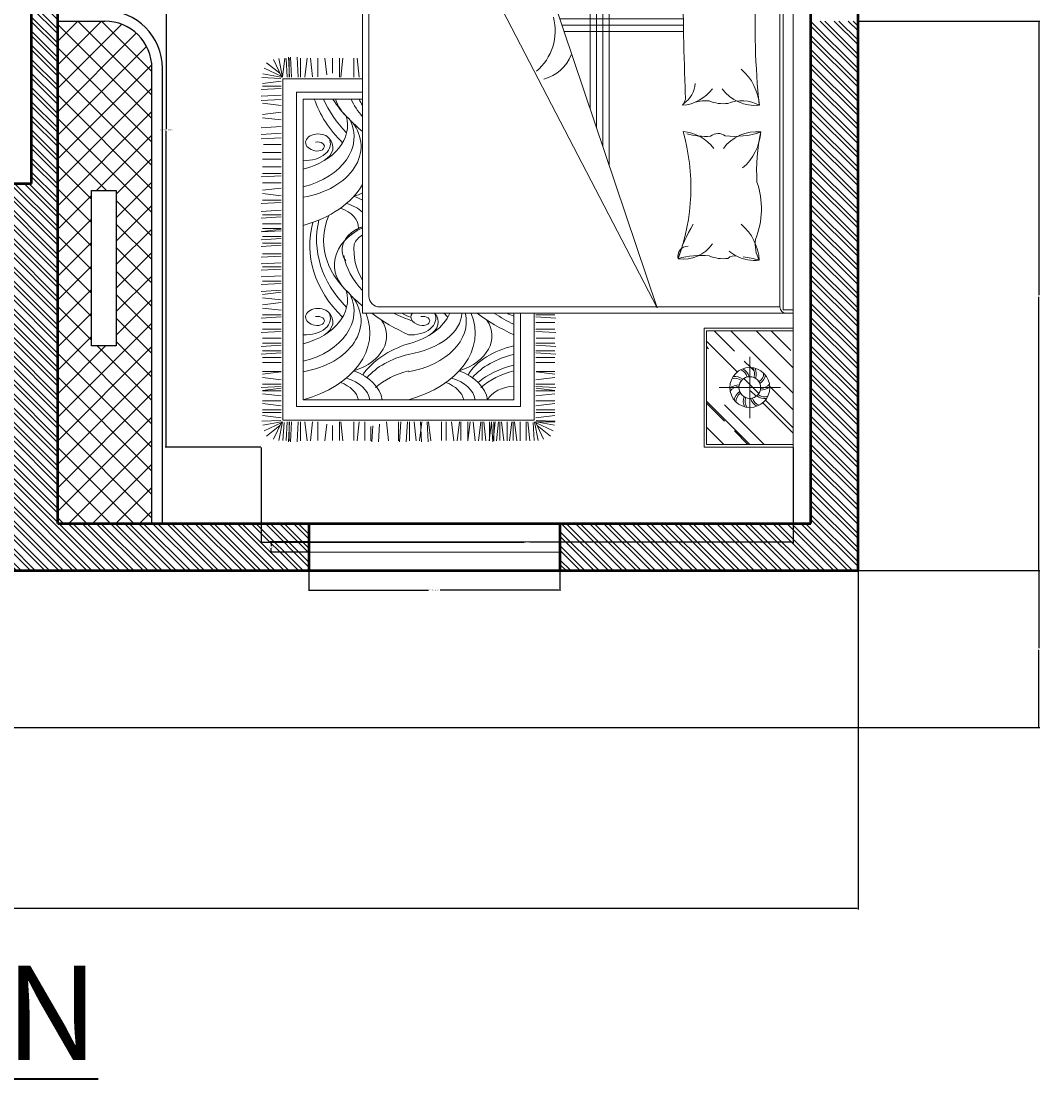
# Model space of a CAD drawing. Units: inches. Extents: x 10696 to 11614, y 5787 to 6498.
# Tile 2 of 9: x 10898 to 11093, y 5790 to 5992. Entities that reach past the tile are written whole.
import ezdxf

# ---------------------------------------------------------------- set-up
doc = ezdxf.new("R2010")
doc.units = ezdxf.units.IN
for name, color, linetype, lineweight in [('A-ANNO-DIMS', 2, 'Continuous', 18), ('A-ANNO-TITL', 7, 'Continuous', 35), ('A-FLOR-CASE', 32, 'Continuous', 25), ('A-FLOR-CASE-PATT', 252, 'Continuous', 13), ('A-FURN', 8, 'Continuous', 18), ('A-GLAZ', 4, 'Continuous', 20), ('A-WALL', 7, 'Continuous', 50), ('A-WALL-PATT', 252, 'Continuous', 13)]:
    doc.layers.add(name, color=color, linetype=linetype, lineweight=lineweight)
doc.styles.get("Standard").update_dxf_attribs({"font": 'arial.ttf'})
doc.dimstyles.get("Standard").update_dxf_attribs({"dimtxt": 0.18, "dimasz": 0.18, "dimexe": 0.18, "dimexo": 0.0625, "dimgap": 0.09, "dimtad": 0, "dimtih": 1, "dimtoh": 1, "dimdec": 4, "dimzin": 0, "dimdsep": 46, "dimtxsty": 'Standard', "dimcen": 0.09, "dimadec": 0, "dimazin": 0, "dimtfac": 1, "dimtdec": 4, "dimtofl": 0, "dimtmove": 0, "dimatfit": 3, "dimfxl": 1, "dimtolj": 1, "dimtzin": 0, "dimarcsym": 0})

# ---------------------------------------------------------------- blocks, each defined once
blk = doc.blocks.new('A$C64B41DC1')
for p, q in [((0, 2.5079), (2.9903, 2.5079)), ((0, 2.0879), (0, 2.5079)), ((0.012, 2.4618), (0.0581, 2.5079)), ((0.012, 2.3515), (0.1684, 2.5079)), ((0.012, 2.0999), (0.012, 2.5079)), ((0.0543, 2.2213), (0.3409, 2.5079)), ((0.1689, 2.4179), (0.2589, 2.5079)), ((0.3265, 2.386), (0.4484, 2.5079)), ((0.3699, 2.3332), (0.5445, 2.5079)), ((0.548, 2.5079), (0.548, 2.0999)), ((0.56, 2.5079), (0.56, 2.0879)), ((0.6301, 2.5079), (0.6301, 0.4779)), ((0.6401, 2.461), (0.6401, 2.5079)), ((0.6401, 2.5079), (2.344, 2.5079)), ((2.344, 2.5079), (2.3601, 2.5079)), ((2.344, 2.5079), (2.344, 2.461)), ((2.3601, 2.5079), (2.3601, 2.4761)), ((2.3601, 0.4779), (2.3601, 2.5079)), ((2.4303, 2.5079), (2.4303, 2.0879)), ((2.4423, 2.5079), (2.4423, 2.0999)), ((2.4423, 2.3333), (2.6169, 2.5079)), ((2.4423, 2.2145), (2.7357, 2.5079)), ((2.4423, 2.404), (2.5354, 2.4971)), ((2.705, 2.398), (2.8149, 2.5079)), ((2.7691, 2.3772), (2.8998, 2.5079)), ((2.7819, 2.3646), (2.9252, 2.5079)), ((2.9783, 2.0999), (2.9783, 2.5079)), ((2.9903, 2.0879), (2.9903, 2.5079)), ((0.2804, 2.1597), (0.2804, 2.4481)), ((2.344, 2.461), (0.6401, 2.461)), ((0.6601, 2.4461), (1.4951, 2.4461)), ((0.6601, 2.4461), (0.6601, 0.5579)), ((1.4951, 2.4461), (0.6697, 2.4461)), ((2.3301, 2.4461), (1.4951, 2.4461)), ((2.3301, 0.5579), (2.3301, 2.4461)), ((2.7099, 2.1597), (2.7099, 2.4481)), ((0.2157, 2.0999), (0.548, 2.4322)), ((0.2299, 2.0999), (0.548, 2.418)), ((0.2311, 2.2906), (0.2937, 2.3532)), ((2.6674, 2.2756), (2.7382, 2.3464)), ((2.7914, 2.1846), (2.9783, 2.3715)), ((0.1362, 2.3039), (0.4246, 2.3039)), ((0.2905, 2.2539), (0.3304, 2.2938)), ((0.3405, 2.3039), (0.3605, 2.3238)), ((2.8541, 2.3039), (2.5657, 2.3039)), ((2.5849, 2.2779), (2.6158, 2.3088)), ((2.6158, 2.3088), (2.6313, 2.3243)), ((2.7249, 2.3076), (2.7512, 2.3339)), ((2.7746, 2.0999), (2.9783, 2.3036)), ((2.9144, 2.2312), (2.9783, 2.2951)), ((0.012, 2.261), (0.0275, 2.2765)), ((0.0404, 2.0999), (0.1982, 2.2578)), ((2.4918, 2.0999), (2.6366, 2.2447)), ((0.1365, 2.0999), (0.251, 2.2144)), ((0.4194, 2.0999), (0.548, 2.2285)), ((2.4423, 2.1353), (2.5382, 2.2312)), ((0.4986, 2.0999), (0.548, 2.1493)), ((2.7831, 2.0999), (2.8678, 2.1846)), ((2.8962, 2.0999), (2.9783, 2.182)), ((0.548, 2.0999), (0.012, 2.0999)), ((0.5127, 2.0999), (0.548, 2.1352)), ((2.4423, 2.0999), (2.9783, 2.0999)), ((2.5172, 2.0999), (2.5269, 2.1096)), ((0.56, 2.0879), (0, 2.0879)), ((2.4303, 2.0879), (2.9903, 2.0879)), ((0.9415, 1.9902), (0.9415, 1.3975)), ((0.9715, 1.9906), (0.9715, 1.4076)), ((1.0015, 1.991), (1.0015, 1.4177)), ((1.0315, 1.9916), (1.0315, 1.4279)), ((2.3349, 1.8678), (0.6613, 1.3029)), ((0.8956, 1.1191), (2.3349, 1.8678)), ((1.6636, 1.6412), (0.6601, 1.6412)), ((1.5748, 1.6112), (0.6601, 1.6112)), ((2.3665, 1.295), (2.3665, 1.3839)), ((2.377, 1.295), (2.3822, 1.3891)), ((2.4032, 1.295), (2.4032, 1.3839)), ((2.4346, 1.295), (2.4346, 1.3839)), ((2.4451, 1.295), (2.4503, 1.3891)), ((2.4774, 1.2957), (2.4774, 1.3837)), ((2.5, 1.295), (2.5, 1.3839)), ((2.5105, 1.295), (2.5157, 1.3891)), ((2.5367, 1.295), (2.5367, 1.3839)), ((2.5471, 1.295), (2.5524, 1.3891)), ((2.5681, 1.295), (2.5681, 1.3839)), ((2.5918, 1.295), (2.5918, 1.3839)), ((2.6346, 1.2957), (2.6346, 1.3837)), ((2.6362, 1.2957), (2.6467, 1.3839)), ((2.6729, 1.295), (2.6624, 1.3839)), ((2.6938, 1.295), (2.6938, 1.3839)), ((2.7043, 1.295), (2.7095, 1.3891)), ((2.7127, 1.2957), (2.7232, 1.3839)), ((2.7253, 1.295), (2.7253, 1.3839)), ((2.7494, 1.295), (2.7389, 1.3839)), ((2.7718, 1.295), (2.7718, 1.3839)), ((2.7959, 1.295), (2.7854, 1.3839)), ((2.8146, 1.2957), (2.8146, 1.3837)), ((2.8146, 1.2957), (2.8146, 1.3837)), ((2.8282, 1.295), (2.8282, 1.3839)), ((2.8282, 1.295), (2.8282, 1.3839)), ((2.8523, 1.295), (2.8418, 1.3839)), ((2.8523, 1.295), (2.8418, 1.3839)), ((2.8653, 1.2966), (2.8688, 1.3861)), ((2.8711, 1.2957), (2.8711, 1.3837)), ((2.8711, 1.2957), (2.8875, 1.3822)), ((2.8765, 1.2958), (2.9132, 1.3758)), ((2.8893, 1.3011), (2.9394, 1.3636)), ((2.8713, 1.2927), (2.954, 1.3315)), ((2.8717, 1.2884), (2.9588, 1.3058)), ((2.3601, 1.2873), (2.8639, 1.2873)), ((2.8639, 1.2873), (2.8639, 0.1018)), ((2.8716, 1.2565), (2.9605, 1.2669)), ((2.8723, 1.2489), (2.9603, 1.2489)), ((2.8744, 1.2817), (2.9603, 1.2869)), ((2.3601, 1.2233), (2.7999, 1.2233)), ((2.7999, 1.2233), (2.7999, 0.1658)), ((2.8716, 1.2212), (2.9605, 1.2212)), ((2.8716, 1.1947), (2.9605, 1.2052)), ((2.3601, 1.1913), (2.7679, 1.1912)), ((2.7679, 1.1912), (2.7679, 0.1978)), ((2.8716, 1.181), (2.9605, 1.1705)), ((2.8716, 1.1595), (2.9605, 1.1595)), ((2.8723, 1.1872), (2.9603, 1.1872)), ((2.8716, 1.133), (2.9605, 1.1435)), ((2.8716, 1.1193), (2.9605, 1.1088)), ((2.8716, 1.1035), (2.9605, 1.093)), ((2.8723, 1.1255), (2.9603, 1.1255)), ((2.8716, 1.0965), (2.9605, 1.0965)), ((2.8716, 1.086), (2.9657, 1.0913)), ((2.8716, 1.0756), (2.9605, 1.0756)), ((2.8716, 1.0491), (2.9605, 1.0596)), ((2.8723, 1.0858), (2.9605, 1.0753)), ((2.8716, 1.0354), (2.9605, 1.0249)), ((2.8723, 1.0416), (2.9603, 1.0416)), ((2.8723, 0.9987), (2.9605, 1.0092)), ((2.8723, 0.985), (2.9605, 0.9745)), ((2.8723, 0.9735), (2.9603, 0.9735)), ((2.8716, 0.9346), (2.9605, 0.9241)), ((2.8723, 0.9408), (2.9603, 0.9408)), ((2.8723, 0.8979), (2.9605, 0.9084)), ((2.8723, 0.8726), (2.9603, 0.8726)), ((2.8723, 0.8505), (2.9603, 0.8505)), ((2.8716, 0.7885), (2.9605, 0.799)), ((2.8716, 0.7818), (2.9657, 0.787)), ((2.8716, 0.7503), (2.9657, 0.7556)), ((2.8723, 0.7571), (2.9605, 0.7466)), ((2.8716, 0.7204), (2.9605, 0.7309)), ((2.8716, 0.6995), (2.9605, 0.6995)), ((2.8716, 0.689), (2.9657, 0.6838)), ((2.8716, 0.6576), (2.9657, 0.6523)), ((2.8716, 0.6471), (2.9605, 0.6471)), ((2.8716, 0.5903), (2.9605, 0.6007)), ((2.882, 0.5582), (2.9657, 0.5536)), ((0.7101, 0.5079), (2.2801, 0.5079)), ((2.8909, 0.5263), (2.9657, 0.5222)), ((2.8928, 0.5169), (2.9605, 0.5169)), ((0.6301, 0.4779), (2.3601, 0.4779)), ((1.2465, 0.4625), (1.1576, 0.452)), ((1.2542, 0.1018), (1.2542, 0.4779)), ((1.3182, 0.1658), (1.3182, 0.4779)), ((1.3502, 0.1978), (1.3502, 0.4779)), ((2.8716, 0.4877), (2.9603, 0.4877)), ((2.8716, 0.4625), (2.9605, 0.452)), ((1.2465, 0.4365), (1.1577, 0.4365)), ((2.8716, 0.4365), (2.9603, 0.4365)), ((1.2465, 0.3746), (1.1576, 0.3851)), ((1.2465, 0.3684), (1.1577, 0.3684)), ((2.8716, 0.3746), (2.9605, 0.3851)), ((2.8716, 0.3684), (2.9603, 0.3684)), ((1.2355, 0.3092), (1.1576, 0.3)), ((1.2285, 0.3357), (1.1577, 0.3357)), ((2.8826, 0.3092), (2.9605, 0.3)), ((2.8896, 0.3357), (2.9603, 0.3357)), ((1.2457, 0.2676), (1.1577, 0.2676)), ((2.8723, 0.2676), (2.9603, 0.2676)), ((1.2457, 0.2423), (1.1576, 0.2319)), ((1.2465, 0.2057), (1.1576, 0.2161)), ((2.8716, 0.2057), (2.9605, 0.2161)), ((2.8723, 0.2423), (2.9605, 0.2319)), ((1.2465, 0.1742), (1.1524, 0.169)), ((1.2465, 0.1847), (1.1576, 0.1847)), ((2.7999, 0.1658), (1.3182, 0.1658)), ((2.7679, 0.1978), (1.3502, 0.1978)), ((2.8716, 0.1847), (2.9605, 0.1847)), ((2.8716, 0.1742), (2.9657, 0.169)), ((1.2465, 0.1428), (1.1524, 0.1376)), ((1.2465, 0.1334), (1.1524, 0.1281)), ((1.2465, 0.1323), (1.1576, 0.1323)), ((1.2465, 0.1323), (1.1576, 0.1323)), ((1.2465, 0.1), (1.1576, 0.1105)), ((1.2465, 0.1229), (1.1588, 0.1168)), ((1.2464, 0.1007), (1.1592, 0.0833)), ((2.8639, 0.1018), (1.2542, 0.1018)), ((2.8716, 0.1428), (2.9657, 0.1376)), ((2.8716, 0.1334), (2.9657, 0.1281)), ((2.8716, 0.1323), (2.9605, 0.1323)), ((2.8716, 0.1229), (2.9593, 0.1168)), ((2.8717, 0.1007), (2.9588, 0.0833)), ((2.8744, 0.1074), (2.9603, 0.1022)), ((1.2468, 0.0964), (1.1641, 0.0576)), ((1.2288, 0.088), (1.1787, 0.0255)), ((1.2415, 0.0933), (1.2049, 0.0133)), ((1.247, 0.0934), (1.2306, 0.0069)), ((1.2527, 0.0925), (1.2493, 0.003)), ((1.2658, 0.0941), (1.2762, 0.0052)), ((1.2899, 0.0941), (1.2899, 0.0052)), ((1.2999, 0.0941), (1.3051, 0)), ((1.3313, 0.0941), (1.3365, 0)), ((1.3523, 0.0941), (1.3575, 0)), ((1.3804, 0.0941), (1.3699, 0.0052)), ((1.4119, 0.0934), (1.4223, 0.0052)), ((1.4485, 0.0941), (1.438, 0.0052)), ((1.48, 0.0941), (1.4852, 0)), ((1.5114, 0.0941), (1.5166, 0)), ((1.5323, 0.0941), (1.5376, 0)), ((1.5638, 0.0941), (1.5638, 0.0105)), ((1.6021, 0.0941), (1.6021, 0.0052)), ((1.6336, 0.0941), (1.6336, 0.0052)), ((1.6702, 0.0941), (1.6702, 0.0052)), ((1.7017, 0.0941), (1.7017, 0.0052)), ((1.7122, 0.0941), (1.7174, 0)), ((1.7445, 0.0934), (1.7445, 0.0054)), ((1.7698, 0.0934), (1.7803, 0.0052)), ((1.8065, 0.0941), (1.796, 0.0052)), ((1.8274, 0.0941), (1.8274, 0.0052)), ((1.8379, 0.0941), (1.8431, 0)), ((1.8746, 0.0941), (1.8798, 0)), ((1.8955, 0.0941), (1.8955, 0.0052)), ((1.906, 0.0941), (1.9113, 0)), ((1.9384, 0.0934), (1.9384, 0.0054)), ((1.9609, 0.0941), (1.9609, 0.0052)), ((1.9636, 0.0934), (1.9741, 0.0052)), ((1.9714, 0.0941), (1.9766, 0)), ((1.9976, 0.0941), (1.9976, 0.0052)), ((2.0081, 0.0941), (2.0133, 0)), ((2.029, 0.0941), (2.029, 0.0052)), ((2.0395, 0.0941), (2.0447, 0)), ((2.0797, 0.0941), (2.0797, 0.0052)), ((2.0902, 0.0941), (2.0954, 0)), ((2.1216, 0.0941), (2.1269, 0)), ((2.1412, 0.0941), (2.1412, 0.0052)), ((2.1517, 0.0941), (2.1569, 0)), ((2.1831, 0.0941), (2.1884, 0)), ((2.2093, 0.0941), (2.2093, 0.0052)), ((2.2198, 0.0941), (2.225, 0)), ((2.2512, 0.0941), (2.2565, 0)), ((2.2603, 0.0934), (2.2707, 0.0052)), ((2.2969, 0.0941), (2.2864, 0.0052)), ((2.3089, 0.0934), (2.3193, 0.0052)), ((2.3455, 0.0941), (2.3351, 0.0052)), ((2.3665, 0.0941), (2.3665, 0.0052)), ((2.377, 0.0941), (2.3822, 0)), ((2.4032, 0.0941), (2.4032, 0.0052)), ((2.4346, 0.0941), (2.4346, 0.0052)), ((2.4451, 0.0941), (2.4503, 0)), ((2.4774, 0.0934), (2.4774, 0.0054)), ((2.5, 0.0941), (2.5, 0.0052)), ((2.5105, 0.0941), (2.5157, 0)), ((2.5367, 0.0941), (2.5367, 0.0052)), ((2.5471, 0.0941), (2.5524, 0)), ((2.5681, 0.0941), (2.5681, 0.0052)), ((2.5918, 0.0941), (2.5918, 0.0052)), ((2.6346, 0.0934), (2.6346, 0.0054)), ((2.6362, 0.0934), (2.6467, 0.0052)), ((2.6729, 0.0941), (2.6624, 0.0052)), ((2.6938, 0.0941), (2.6938, 0.0052)), ((2.7043, 0.0941), (2.7095, 0)), ((2.7127, 0.0934), (2.7232, 0.0052)), ((2.7253, 0.0941), (2.7253, 0.0052)), ((2.7494, 0.0941), (2.7389, 0.0052)), ((2.7718, 0.0941), (2.7718, 0.0052)), ((2.7959, 0.0941), (2.7854, 0.0052)), ((2.8146, 0.0934), (2.8146, 0.0054)), ((2.8282, 0.0941), (2.8282, 0.0052)), ((2.8523, 0.0941), (2.8418, 0.0052)), ((2.8653, 0.0925), (2.8688, 0.003)), ((2.8711, 0.0934), (2.8875, 0.0069)), ((2.8713, 0.0964), (2.954, 0.0576)), ((2.8765, 0.0933), (2.9132, 0.0133)), ((2.8893, 0.088), (2.9394, 0.0255))]:
    blk.add_line(p, q)
at = {"ltscale": 10}
for p, q in [((1.4859, 1.5812), (0.6601, 1.5812)), ((1.397, 1.5512), (0.6601, 1.5512))]:
    blk.add_line(p, q, dxfattribs=at)
for centre, radius in [((0.2804, 2.3039), 0.0942), ((2.7099, 2.3039), 0.0942), ((0.2804, 2.3039), 0.051), ((2.7099, 2.3039), 0.051)]:
    blk.add_circle(centre, radius)
for centre, radius, start, end in [((0.6601, 2.4761), 0.03, 180, 270), ((2.3301, 2.4761), 0.03, 270, 0), ((0.3286, 2.3561), 0.0605, 136.17, 182.4897), ((0.3231, 2.3585), 0.0462, 124.3002, 184.538), ((2.6672, 2.3585), 0.0462, 355.462, 55.6998), ((2.6617, 2.3561), 0.0605, 357.5103, 43.83), ((0.2417, 2.3614), 0.0462, 196.3002, 256.538), ((0.2887, 2.3745), 0.0605, 172.17, 218.4897), ((0.2828, 2.3731), 0.0462, 160.3002, 220.538), ((0.3501, 2.3178), 0.0605, 100.17, 146.4897), ((0.347, 2.323), 0.0462, 88.3002, 148.538), ((1.0526, 2.3302), 0.3085, 175.3048, 198.6942), ((-0.8702, 2.0941), 1.6364, 4.8098, 9.1892), ((0.8579, 2.6278), 0.2948, 247.5179, 264.267), ((0.728, 2.111), 0.245, 40.4189, 85.9871), ((1.0164, 5.7096), 3.3803, 266.8134, 276.1602), ((1.3963, 2.1044), 0.245, 94.0129, 139.5811), ((1.1858, 2.3288), 0.1943, 306.5711, 5.89), ((1.5348, 2.2652), 0.1767, 151.7736, 201.6983), ((1.6986, 2.3355), 0.1943, 174.11, 233.4289), ((1.1481, 2.2311), 0.3783, 353.4947, 19.1867), ((1.6871, 3.192), 0.8561, 257.7438, 273.6284), ((1.4882, 2.111), 0.245, 40.4189, 85.9871), ((1.8674, 1.9709), 0.3878, 68.2026, 108.9817), ((2.1269, 2.1044), 0.245, 94.0129, 139.5811), ((2.0342, 2.4856), 0.1563, 261.5958, 298.9092), ((1.9165, 2.3288), 0.1943, 333.7371, 5.89), ((2.6058, 2.2028), 0.517, 163.6046, 172.3273), ((2.6433, 2.323), 0.0462, 31.462, 91.6998), ((2.6402, 2.3178), 0.0605, 33.5103, 79.83), ((2.7075, 2.3731), 0.0462, 319.462, 19.6998), ((2.7016, 2.3745), 0.0605, 321.5103, 7.83), ((2.7486, 2.3614), 0.0462, 283.462, 343.6998), ((0.2457, 2.3659), 0.0605, 208.17, 254.4897), ((0.3449, 2.2742), 0.0605, 64.17, 110.4897), ((0.3455, 2.2802), 0.0462, 52.3002, 112.538), ((0.3151, 2.2419), 0.0605, 28.17, 74.4897), ((2.6448, 2.2802), 0.0462, 67.462, 127.6998), ((2.6454, 2.2742), 0.0605, 69.5103, 115.83), ((2.6752, 2.2419), 0.0605, 105.5103, 151.83), ((2.7446, 2.3659), 0.0605, 285.5103, 331.83), ((0.2153, 2.3276), 0.0462, 232.3002, 292.538), ((0.2158, 2.3336), 0.0605, 244.17, 290.4897), ((0.2138, 2.2848), 0.0462, 268.3002, 328.538), ((0.2107, 2.29), 0.0605, 280.17, 326.4897), ((0.2377, 2.2493), 0.0462, 304.3002, 4.538), ((0.2322, 2.2517), 0.0605, 316.17, 2.4897), ((0.2779, 2.2347), 0.0462, 340.3002, 40.538), ((0.272, 2.2333), 0.0605, 352.17, 38.4897), ((0.3191, 2.2464), 0.0462, 16.3002, 76.538), ((2.6712, 2.2464), 0.0462, 103.462, 163.6998), ((2.7182, 2.2333), 0.0605, 141.5103, 187.83), ((2.7123, 2.2347), 0.0462, 139.462, 199.6998), ((2.7581, 2.2517), 0.0605, 177.5103, 223.83), ((2.7526, 2.2493), 0.0462, 175.462, 235.6998), ((2.7796, 2.29), 0.0605, 213.5103, 259.83), ((2.7765, 2.2848), 0.0462, 211.462, 271.6998), ((2.7744, 2.3336), 0.0605, 249.5103, 295.83), ((2.775, 2.3276), 0.0462, 247.462, 307.6998), ((0.7274, 2.2013), 0.0446, 314.4736, 42.1713), ((-1.6008, 2.277), 2.3618, 357.3905, 358.8876), ((1.204, 2.1778), 0.1681, 337.017, 7.5368), ((1.9165, 2.3288), 0.1943, 320.9404, 333.7371), ((2.1347, 2.2313), 0.0459, 165.3506, 223.2684), ((1.9346, 2.1778), 0.1681, 337.017, 7.5368), ((0.2688, 2.0945), 0.4956, 344.0243, 8.7071), ((1.5671, 2.1546), 0.0547, 142.0833, 220.902), ((0.9385, 1.978), 0.1943, 126.5711, 185.89), ((1.1858, 1.9714), 0.1943, 4.3181, 53.4289), ((1.5415, 2.0969), 0.1834, 175.2233, 196.23), ((1.7059, 1.9714), 0.204, 127.1197, 175.09), ((1.1965, 2.0983), 0.3299, 343.7954, 3.5554), ((1.9394, 1.991), 0.1651, 351.2621, 55.7572), ((2.4617, 2.0719), 0.3745, 173.8296, 196.4356), ((1.2687, 1.9248), 0.1223, 33.628, 86.4744), ((0.7246, 18.8439), 16.8552, 270.17399, 272.05214), ((1.3401, 1.9404), 0.0603, 49.0991, 101.3702), ((1.7676, 1.0629), 0.9631, 69.6507, 105.9631), ((2.2748, 2.5795), 0.6373, 238.3499, 254.3137), ((2.0911, 2.0123), 0.0478, 179.7727, 283.8018), ((0.7417, 2.0149), 0.057, 273.4709, 328.5412), ((0.728, 2.2025), 0.245, 274.0129, 278.3417), ((1.0747, 1.2871), 0.1871, 14.1863, 69.1212), ((1.0274, 1.1334), 0.2527, 40.629, 104.3712), ((0.7347, 1.1553), 0.1649, 347.3109, 116.4454), ((0.7101, 0.5579), 0.05, 180, 270), ((2.2801, 0.5579), 0.05, 270, 0)]:
    blk.add_arc(centre, radius, start, end)
for centre, major_axis, ratio, start_param, end_param in [((1.9938, 1.6262), (0, -0.7531), 0.68, 0.797284, 0.954936), ((2.0643, 1.466), (0, -0.5322), 0.68, 7.239912, 7.311536), ((1.9052, 1.7397), (0, -0.9842), 0.68, 0.74745, 0.979724), ((2.7455, 1.3081), (0, 0.3614), 0.68, 1.900046, 2.742661), ((2.7868, 1.3081), (0, 0.3614), 0.68, 1.900046, 2.614747), ((2.8372, 1.3081), (0, 0.3614), 0.68, 1.900046, 2.479658), ((2.8607, 1.3211), (0, 0.3614), 0.68, 1.938265, 2.479658), ((2.8057, 1.2079), (0, -0.1524), 0.68, 4.821745, 5.895886), ((2.4665, 0.8216), (0, -0.2664), 0.68, 2.006169, 3.565187), ((2.4513, 0.5069), (0, 0.502), 0.68, 5.095327, 6.553458), ((2.7862, 0.8069), (0, -0.2615), 0.68, 3.244645, 4.205018), ((2.7784, 0.8289), (0, -0.1802), 0.68, 3.227058, 4.318474), ((2.396, 0.6032), (0, 0.3641), 0.68, -1.3172, 0.145284), ((2.7821, 0.7971), (0, -0.1589), 0.68, 3.272942, 4.229533), ((2.3507, 0.5642), (0.0073, 0.3819), 0.56205, -1.21172, -0.009991), ((2.2964, 0.5771), (0, -0.3263), 0.68, 1.938944, 2.850232), ((2.0403, 1.6015), (0, -0.8763), 0.68, 6.849801, 6.887077), ((2.4005, 0.7132), (0, -0.1214), 0.68, 2.284368, 3.652258), ((2.3834, 0.7081), (0, 0.1147), 0.68, 4.593909, 6.585576), ((2.3774, 0.7653), (0, -0.0593), 0.68, 5.841311, 7.755362), ((2.3961, 0.7628), (0, -0.0317), 0.68, 1.462497, 5.046281), ((1.9938, 1.1295), (-0.0678, 0.7439), 0.610498, 3.917146, 4.063997), ((2.0643, 0.9693), (0, -0.5322), 0.68, 7.239912, 7.336618), ((1.9052, 1.243), (0, -0.9842), 0.68, 0.74745, 0.979724), ((2.7455, 0.8114), (-0.0599, 0.3735), 0.695517, 1.775813, 2.548612), ((2.7868, 0.8114), (0, 0.3614), 0.68, 1.900046, 2.614747), ((2.8607, 0.8243), (0, 0.3614), 0.68, 1.938265, 2.479658), ((2.4665, 0.3249), (0, -0.2664), 0.68, 2.006169, 3.565187), ((2.4513, 0.0102), (0, 0.502), 0.68, 5.095327, 6.553458), ((2.7862, 0.3102), (0, -0.2615), 0.68, 3.244645, 4.205018), ((2.7784, 0.3322), (0, -0.1802), 0.68, 3.227058, 4.318474), ((1.242, 0.9693), (0, -0.5322), 0.68, 6.586764, 6.677612), ((1.1714, 1.1295), (-0.1157, 0.7241), 0.59432, 3.291697, 3.50733), ((1.0828, 1.243), (0, -0.9842), 0.68, 0.565948, 0.680366), ((1.5283, 0.0674), (0, -0.3703), 0.68, 1.930561, 3.464283), ((1.5736, 0.1065), (0, 0.3641), 0.68, -1.3172, 0.476403), ((1.6289, 0.0102), (0, 0.502), 0.68, 6.655152, 6.661293), ((1.6289, 0.0102), (0, 0.502), 0.68, 5.095327, 5.911219), ((1.6442, 0.3249), (0, -0.2664), 0.68, 2.006169, 2.182797), ((1.9638, 0.3102), (0, -0.2615), 0.68, 4.015924, 4.205018), ((1.956, 0.3322), (0, -0.1802), 0.68, 3.770744, 4.318474), ((1.9597, 0.3004), (0, -0.1589), 0.68, 3.14258, 4.229533), ((2.0606, 0.5616), (0, -0.1803), 0.68, 5.194792, 5.929328), ((2.0606, 0.5616), (0, -0.1803), 0.68, 5.194792, 6.723255), ((2.1315, 0.6603), (0, -0.3155), 0.68, 5.328638, 6.949396), ((2.0549, 0.5656), (0, -0.1303), 0.68, 5.450951, 6.054641), ((2.0643, 0.9693), (0, -0.5322), 0.68, 6.20013, 6.677612), ((1.9938, 1.1295), (-0.0678, 0.7439), 0.610498, 3.199135, 3.592282), ((1.9052, 1.243), (0, -0.9842), 0.68, 0.565948, 0.680366), ((2.3507, 0.0674), (0, -0.3703), 0.68, 1.930561, 3.464283), ((2.396, 0.1065), (0, 0.3641), 0.68, -1.3172, 0.476403), ((2.4513, 0.0102), (0, 0.502), 0.68, 6.655152, 6.661293), ((2.7821, 0.3004), (0, -0.1589), 0.68, 3.272942, 4.229533), ((1.1933, 0.9181), (0, -0.624), 0.68, 0.378672, 0.625379), ((1.3091, 0.6603), (0, -0.3155), 0.68, 6.475719, 6.949396), ((1.1911, 1.1066), (0, 0.8458), 0.68, 3.421828, 3.728616), ((1.474, 0.0804), (0, -0.3263), 0.68, 1.938944, 3.339184), ((2.0157, 0.9181), (0, -0.624), 0.68, -0.280078, 0.625379), ((2.0135, 1.1066), (0, 0.8458), 0.68, 2.978727, 3.728616), ((2.2964, 0.0804), (0, -0.3263), 0.68, 1.938944, 3.339184), ((1.2179, 1.1047), (0, -0.8763), 0.68, 6.507006, 6.887077), ((1.5781, 0.2165), (0, -0.1214), 0.68, 2.284368, 3.726131), ((2.0403, 1.1047), (0, -0.8763), 0.68, 6.099302, 6.887077), ((2.4005, 0.2165), (0, -0.1214), 0.68, 2.284368, 3.726131), ((1.555, 0.2685), (0, -0.0593), 0.68, 3.732151, 7.755362), ((1.561, 0.2114), (0, 0.1147), 0.68, 4.593909, 6.647252), ((1.5737, 0.2661), (0, -0.0317), 0.68, 1.462497, 5.046281), ((2.3774, 0.2685), (0, -0.0593), 0.68, 3.732151, 7.755362), ((2.3834, 0.2114), (0, 0.1147), 0.68, 4.593909, 6.647252), ((2.3961, 0.2661), (0, -0.0317), 0.68, 1.462497, 5.046281)]:
    blk.add_ellipse(centre, major_axis=major_axis, ratio=ratio, start_param=start_param, end_param=end_param)
blk = doc.blocks.new('WIN-GLAZ-48')
for p, q in [((0, 48), (0, 0)), ((2, 48), (2, 0))]:
    blk.add_line(p, q)
blk = doc.blocks.new('*D28')
at = {"layer": 'A-ANNO-DIMS', "color": 0, "lineweight": -2, "transparency": 16777216}
for p, q in [((10952.91, 5890.51), (10952.91, 5883.19)), ((11000.91, 5890.51), (11000.91, 5883.19)), ((10953.09, 5883.37), (10975.79, 5883.37)), ((11000.73, 5883.37), (10978.03, 5883.37))]:
    blk.add_line(p, q, dxfattribs=at)
at = {"layer": 'A-ANNO-DIMS', "color": 0, "transparency": 16777216}
for points in [[(10953.09, 5883.4), (10953.09, 5883.34), (10952.91, 5883.37)], [(11000.73, 5883.4), (11000.73, 5883.34), (11000.91, 5883.37)]]:
    blk.add_solid(points, dxfattribs=at)
at = {"layer": 'Defpoints', "color": 0, "transparency": 16777216}
for p in [(10952.91, 5890.57), (11000.91, 5890.57), (11000.91, 5883.37)]:
    blk.add_point(p, dxfattribs=at)
at = {"layer": 'A-ANNO-DIMS', "color": 0, "transparency": 16777216, "insert": (10976.91, 5883.37), "char_height": 0.18, "attachment_point": 5}
blk.add_mtext('\\A1;WINDOW 48 TYP.', dxfattribs=at)
blk = doc.blocks.new('*D29')
at = {"layer": 'A-ANNO-DIMS', "color": 0, "lineweight": -2, "transparency": 16777216}
for p, q in [((10952.85, 5892.57), (10945.53, 5892.57)), ((10945.71, 5892.39), (10945.71, 5891.75)), ((10952.85, 5890.57), (10945.53, 5890.57)), ((10945.71, 5890.75), (10945.71, 5891.39))]:
    blk.add_line(p, q, dxfattribs=at)
at = {"layer": 'A-ANNO-DIMS', "color": 0, "transparency": 16777216}
for points in [[(10945.68, 5892.39), (10945.74, 5892.39), (10945.71, 5892.57)], [(10945.68, 5890.75), (10945.74, 5890.75), (10945.71, 5890.57)]]:
    blk.add_solid(points, dxfattribs=at)
at = {"layer": 'Defpoints', "color": 0, "transparency": 16777216}
for p in [(10952.91, 5892.57), (10945.71, 5890.57), (10952.91, 5890.57)]:
    blk.add_point(p, dxfattribs=at)
at = {"layer": 'A-ANNO-DIMS', "color": 0, "transparency": 16777216, "insert": (10945.71, 5891.57), "char_height": 0.18, "attachment_point": 5}
blk.add_mtext('\\A1;2 TYP.', dxfattribs=at)
blk = doc.blocks.new('*D42')
at = {"layer": 'A-ANNO-DIMS', "color": 0, "lineweight": -2, "transparency": 16777216}
for p, q in [((10943.75, 6031.92), (10925.45, 6031.92)), ((10925.63, 6031.74), (10925.63, 5971.49)), ((10925.63, 5910.87), (10925.63, 5971.12)), ((10943.75, 5910.69), (10925.45, 5910.69))]:
    blk.add_line(p, q, dxfattribs=at)
at = {"layer": 'A-ANNO-DIMS', "color": 0, "transparency": 16777216}
for points in [[(10925.6, 6031.74), (10925.66, 6031.74), (10925.63, 6031.92)], [(10925.6, 5910.87), (10925.66, 5910.87), (10925.63, 5910.69)]]:
    blk.add_solid(points, dxfattribs=at)
at = {"layer": 'Defpoints', "color": 0, "transparency": 16777216}
for p in [(10943.82, 6031.92), (10925.63, 5910.69), (10943.82, 5910.69)]:
    blk.add_point(p, dxfattribs=at)
at = {"layer": 'A-ANNO-DIMS', "color": 0, "transparency": 16777216, "insert": (10925.63, 5971.31), "char_height": 0.18, "attachment_point": 5}
blk.add_mtext('\\A1;BED GROUP 121 TYP.', dxfattribs=at)
blk = doc.blocks.new('*D43')
at = {"layer": 'A-ANNO-DIMS', "color": 0, "lineweight": -2, "transparency": 16777216}
for p, q in [((10943.82, 5910.63), (10943.82, 5892.33)), ((11045.49, 5910.63), (11045.49, 5892.33)), ((10944, 5892.51), (10994.06, 5892.51)), ((11045.31, 5892.51), (10995.24, 5892.51))]:
    blk.add_line(p, q, dxfattribs=at)
at = {"layer": 'A-ANNO-DIMS', "color": 0, "transparency": 16777216}
for points in [[(10944, 5892.54), (10944, 5892.48), (10943.82, 5892.51)], [(11045.31, 5892.54), (11045.31, 5892.48), (11045.49, 5892.51)]]:
    blk.add_solid(points, dxfattribs=at)
at = {"layer": 'Defpoints', "color": 0, "transparency": 16777216}
for p in [(10943.82, 5910.69), (11045.49, 5910.69), (11045.49, 5892.51)]:
    blk.add_point(p, dxfattribs=at)
at = {"layer": 'A-ANNO-DIMS', "color": 0, "transparency": 16777216, "insert": (10994.65, 5892.51), "char_height": 0.18, "attachment_point": 5}
blk.add_mtext('\\A1;102 TYP.', dxfattribs=at)
blk = doc.blocks.new('*D70')
at = {"layer": 'A-ANNO-DIMS', "color": 0, "lineweight": -2, "transparency": 16777216}
for p, q in [((10730.91, 5887.01), (10730.91, 5822.34)), ((11057.91, 5887.01), (11057.91, 5822.34)), ((10731.09, 5822.52), (10894.12, 5822.52)), ((11057.73, 5822.52), (10894.7, 5822.52))]:
    blk.add_line(p, q, dxfattribs=at)
at = {"layer": 'A-ANNO-DIMS', "color": 0, "transparency": 16777216}
for points in [[(10731.09, 5822.55), (10731.09, 5822.49), (10730.91, 5822.52)], [(11057.73, 5822.55), (11057.73, 5822.49), (11057.91, 5822.52)]]:
    blk.add_solid(points, dxfattribs=at)
at = {"layer": 'Defpoints', "color": 0, "transparency": 16777216}
for p in [(10730.91, 5887.07), (11057.91, 5887.07), (11057.91, 5822.52)]:
    blk.add_point(p, dxfattribs=at)
at = {"layer": 'A-ANNO-DIMS', "color": 0, "transparency": 16777216, "insert": (10894.41, 5822.52), "char_height": 0.18, "attachment_point": 5}
blk.add_mtext('\\A1;327', dxfattribs=at)
blk = doc.blocks.new('*D74')
at = {"layer": 'A-ANNO-DIMS', "color": 0, "lineweight": -2, "transparency": 16777216}
for p, q in [((10895.98, 5887.07), (11092.64, 5887.07)), ((11092.46, 5886.89), (11092.46, 5872.25)), ((11092.46, 5857.25), (11092.46, 5871.89)), ((10895.98, 5857.07), (11092.64, 5857.07))]:
    blk.add_line(p, q, dxfattribs=at)
at = {"layer": 'A-ANNO-DIMS', "color": 0, "transparency": 16777216}
for points in [[(11092.43, 5886.89), (11092.49, 5886.89), (11092.46, 5887.07)], [(11092.43, 5857.25), (11092.49, 5857.25), (11092.46, 5857.07)]]:
    blk.add_solid(points, dxfattribs=at)
at = {"layer": 'Defpoints', "color": 0, "transparency": 16777216}
for p in [(10895.91, 5887.07), (11092.46, 5887.07), (10895.91, 5857.07)]:
    blk.add_point(p, dxfattribs=at)
at = {"layer": 'A-ANNO-DIMS', "color": 0, "transparency": 16777216, "insert": (11092.46, 5872.07), "char_height": 0.18, "attachment_point": 5}
blk.add_mtext('\\A1;30', dxfattribs=at)
blk = doc.blocks.new('*D87')
at = {"layer": 'A-ANNO-DIMS', "color": 0, "lineweight": -2, "transparency": 16777216}
for p, q in [((11057.98, 5992.07), (11092.64, 5992.07)), ((11092.46, 5991.89), (11092.46, 5939.75)), ((11092.46, 5887.25), (11092.46, 5939.39)), ((11057.98, 5887.07), (11092.64, 5887.07))]:
    blk.add_line(p, q, dxfattribs=at)
at = {"layer": 'A-ANNO-DIMS', "color": 0, "transparency": 16777216}
for points in [[(11092.43, 5991.89), (11092.49, 5991.89), (11092.46, 5992.07)], [(11092.43, 5887.25), (11092.49, 5887.25), (11092.46, 5887.07)]]:
    blk.add_solid(points, dxfattribs=at)
at = {"layer": 'Defpoints', "color": 0, "transparency": 16777216}
for p in [(11057.91, 5992.07), (11092.46, 5992.07), (11057.91, 5887.07)]:
    blk.add_point(p, dxfattribs=at)
at = {"layer": 'A-ANNO-DIMS', "color": 0, "transparency": 16777216, "insert": (11092.46, 5939.57), "char_height": 0.18, "attachment_point": 5}
blk.add_mtext('\\A1;105', dxfattribs=at)

msp = doc.modelspace()

# ---------------------------------------------------------------- hatches: boundary and pattern name
at = {"layer": 'A-FLOR-CASE-PATT'}
h = msp.add_hatch(dxfattribs=at)
h.set_pattern_fill('ANSI37', color=256)
h.paths.add_polyline_path([(10922.913, 5983.07, 0.4142136), (10913.913, 5992.07), (10904.913, 5992.07), (10904.913, 5896.07), (10922.913, 5896.07)])
h.paths.add_polyline_path([(10916.11, 5930.013), (10911.36, 5930.013), (10911.36, 5959.701), (10916.11, 5959.701)], flags=16)
at = {"layer": 'A-WALL-PATT'}
h = msp.add_hatch(dxfattribs=at)
h.set_pattern_fill('ANSI32', color=256, scale=0.2, angle=90)
h.paths.add_polyline_path([(10767.913, 5961.07), (10739.913, 5961.07), (10739.913, 6001.333), (10730.913, 6001.333), (10730.913, 5887.07), (10739.913, 5887.07), (10739.913, 5952.07), (10767.913, 5952.07)])
h.paths.add_polyline_path([(10739.913, 6127.055), (10730.913, 6127.055), (10730.913, 6073.333), (10739.913, 6073.333)])
h.paths.add_polyline_path([(10739.913, 6267.869, -0.035413), (10740.694, 6278.876), (10731.784, 6280.146, 0.035413), (10730.913, 6267.869), (10730.913, 6199.055), (10739.913, 6199.055)])
h.paths.add_polyline_path([(10794.29, 6342.205), (10791.564, 6350.783, 0.1142038), (10757.817, 6330.777), (10764.034, 6324.269, -0.1142038)])
h.paths.add_polyline_path([(10844.262, 6350.783), (10841.536, 6342.205, -0.065871), (10860.057, 6333.503), (10864.919, 6341.077, 0.065871)])
h.paths.add_polyline_path([(10908.913, 6311.07), (10895.913, 6311.07), (10895.913, 6306.404, 0.0519949), (10886.285, 6321.667), (10879.212, 6316.101, -0.1682272), (10895.913, 6267.869), (10895.913, 6223.07), (10904.913, 6223.07), (10904.913, 6302.07), (10908.913, 6302.07)])
h.paths.add_polyline_path([(11057.913, 6311.07), (10944.913, 6311.07), (10944.913, 6302.07), (11048.913, 6302.07), (11048.913, 6273.514), (11057.913, 6273.514)])
h.paths.add_polyline_path([(11057.913, 6225.514), (11048.913, 6225.514), (11048.913, 6187.07), (10988.913, 6187.07), (10988.913, 6182.07), (11048.913, 6182.07), (11048.913, 6164.07), (11057.913, 6164.07)])
h.paths.add_polyline_path([(10952.913, 6187.07), (10895.913, 6187.07), (10895.913, 6182.07), (10948.913, 6182.07), (10948.913, 6113.07), (10952.913, 6113.07), (10952.913, 6117.07), (11048.913, 6117.07), (11048.913, 6099.07), (11057.913, 6099.07), (11057.913, 6140.07), (11048.913, 6140.07), (11048.913, 6122.07), (10952.913, 6122.07)])
h.paths.add_polyline_path([(11057.913, 6075.07), (11048.913, 6075.07), (11048.913, 6057.07), (10952.913, 6057.07), (10952.913, 6083.07), (10944.913, 6083.07), (10944.913, 6078.07), (10948.913, 6078.07), (10948.913, 6052.07), (11048.913, 6052.07), (11048.913, 6028.07), (11057.913, 6028.07)])
h.paths.add_polyline_path([(11057.913, 5992.07), (11048.913, 5992.07), (11048.913, 5896.07), (11000.913, 5896.07), (11000.913, 5887.07), (11057.913, 5887.07)])
h.paths.add_polyline_path([(10952.913, 5896.07), (10904.913, 5896.07), (10904.913, 6078.07), (10908.913, 6078.07), (10908.913, 6083.07), (10899.913, 6083.07), (10899.913, 5961.07), (10891.913, 5961.07), (10891.913, 5952.07), (10895.913, 5952.07), (10895.913, 5887.07), (10952.913, 5887.07)])
h.paths.add_polyline_path([(10843.913, 5961.07), (10815.913, 5961.07), (10815.913, 5952.07), (10843.913, 5952.07)])

# ---------------------------------------------------------------- linework, layer by layer
at = {"layer": 'A-FLOR-CASE'}
for p, q in [((10904.913, 5992.07), (10913.913, 5992.07)), ((10922.913, 5896.07), (10922.913, 5983.07)), ((10924.913, 5896.07), (10924.913, 5983.07))]:
    msp.add_line(p, q, dxfattribs=at)
msp.add_lwpolyline([(10911.36, 5959.701), (10916.11, 5959.701), (10916.11, 5930.013), (10911.36, 5930.013)], close=True, dxfattribs=at)
for radius in [11, 9]:
    msp.add_arc((10913.913, 5983.07), radius, 0, 90, dxfattribs=at)
at = {"layer": 'A-WALL'}
for p, q in [((11057.913, 5887.07), (11057.913, 6311.07)), ((10899.913, 5961.07), (10899.913, 6083.07)), ((10904.913, 5896.07), (10904.913, 6078.07)), ((11048.913, 5896.07), (11048.913, 6052.07)), ((10891.913, 5961.07), (10899.913, 5961.07)), ((10904.913, 5896.07), (11048.913, 5896.07)), ((10952.913, 5896.07), (10952.913, 5887.07)), ((11000.913, 5896.07), (11000.913, 5887.07)), ((10895.913, 5887.07), (11057.913, 5887.07))]:
    msp.add_line(p, q, dxfattribs=at)

# ---------------------------------------------------------------- block references
at = {"layer": 'A-FURN', "xscale": 40.54062585747614, "yscale": 40.54062585747614, "zscale": 40.54062585747614, "rotation": 270}
msp.add_blockref('A$C64B41DC1', (10943.816, 6031.92), dxfattribs=at)
at = {"layer": 'A-GLAZ', "rotation": 269.9999999999979}
msp.add_blockref('WIN-GLAZ-48', (10952.913, 5892.57), dxfattribs=at)

# ---------------------------------------------------------------- texts
at = {"layer": 'A-ANNO-TITL', "insert": (10766.66, 5811.558), "char_height": 18, "attachment_point": 1}
msp.add_mtext_dynamic_manual_height_columns('{\\LFLOOR PLAN}', width=251.84009, gutter_width=12.5, heights=[0], dxfattribs=at)

# ---------------------------------------------------------------- dimensions: what is measured, and where the dimension line sits
at = {"layer": 'A-ANNO-DIMS'}
for base, p1, p2, text, picture, middle in [((10925.632, 5910.692), (10943.816, 6031.92), (10943.816, 5910.692), 'BED GROUP <> TYP.', '*D42', (10925.632, 5971.306)), ((10945.713, 5890.57), (10952.913, 5892.57), (10952.913, 5890.57), '<> TYP.', '*D29', (10945.713, 5891.57))]:
    dim = msp.add_linear_dim(base=base, p1=p1, p2=p2, angle=270, text=text, dimstyle='Standard', override={"dimdec": 0, "dimlfac": 1, "dimrnd": 0, "dimzin": 0, "dimdsep": 46, "dimlunit": 2}, dxfattribs=at)
    dim.commit()
    dim.dimension.update_dxf_attribs({"geometry": picture, "text_midpoint": middle})
for base, p1, p2, picture, middle in [((11092.463, 5992.07), (11057.913, 5887.07), (11057.913, 5992.07), '*D87', (11092.463, 5939.57)), ((11092.463, 5887.07), (10895.913, 5857.07), (10895.913, 5887.07), '*D74', (11092.463, 5872.07))]:
    dim = msp.add_linear_dim(base=base, p1=p1, p2=p2, angle=90, dimstyle='Standard', override={"dimdec": 0, "dimlfac": 1, "dimrnd": 0, "dimzin": 0, "dimdsep": 46, "dimlunit": 2}, dxfattribs=at)
    dim.commit()
    dim.dimension.update_dxf_attribs({"geometry": picture, "text_midpoint": middle})
for base, p1, p2, text, picture, middle in [((11045.488, 5892.508), (10943.816, 5910.692), (11045.488, 5910.692), '<> TYP.', '*D43', (10994.652, 5892.508)), ((11000.913, 5883.37), (10952.913, 5890.57), (11000.913, 5890.57), 'WINDOW <> TYP.', '*D28', (10976.913, 5883.37))]:
    dim = msp.add_linear_dim(base=base, p1=p1, p2=p2, text=text, dimstyle='Standard', override={"dimdec": 0, "dimlfac": 1, "dimrnd": 0, "dimzin": 0, "dimdsep": 46, "dimlunit": 2}, dxfattribs=at)
    dim.commit()
    dim.dimension.update_dxf_attribs({"geometry": picture, "text_midpoint": middle})
dim = msp.add_linear_dim(base=(11057.913, 5822.52), p1=(10730.913, 5887.07), p2=(11057.913, 5887.07), dimstyle='Standard', override={"dimdec": 0, "dimlfac": 1, "dimrnd": 0, "dimzin": 0, "dimdsep": 46, "dimlunit": 2}, dxfattribs=at)
dim.commit()
dim.dimension.update_dxf_attribs({"geometry": '*D70', "text_midpoint": (10894.413, 5822.52)})

doc.saveas('drawing.dxf')
